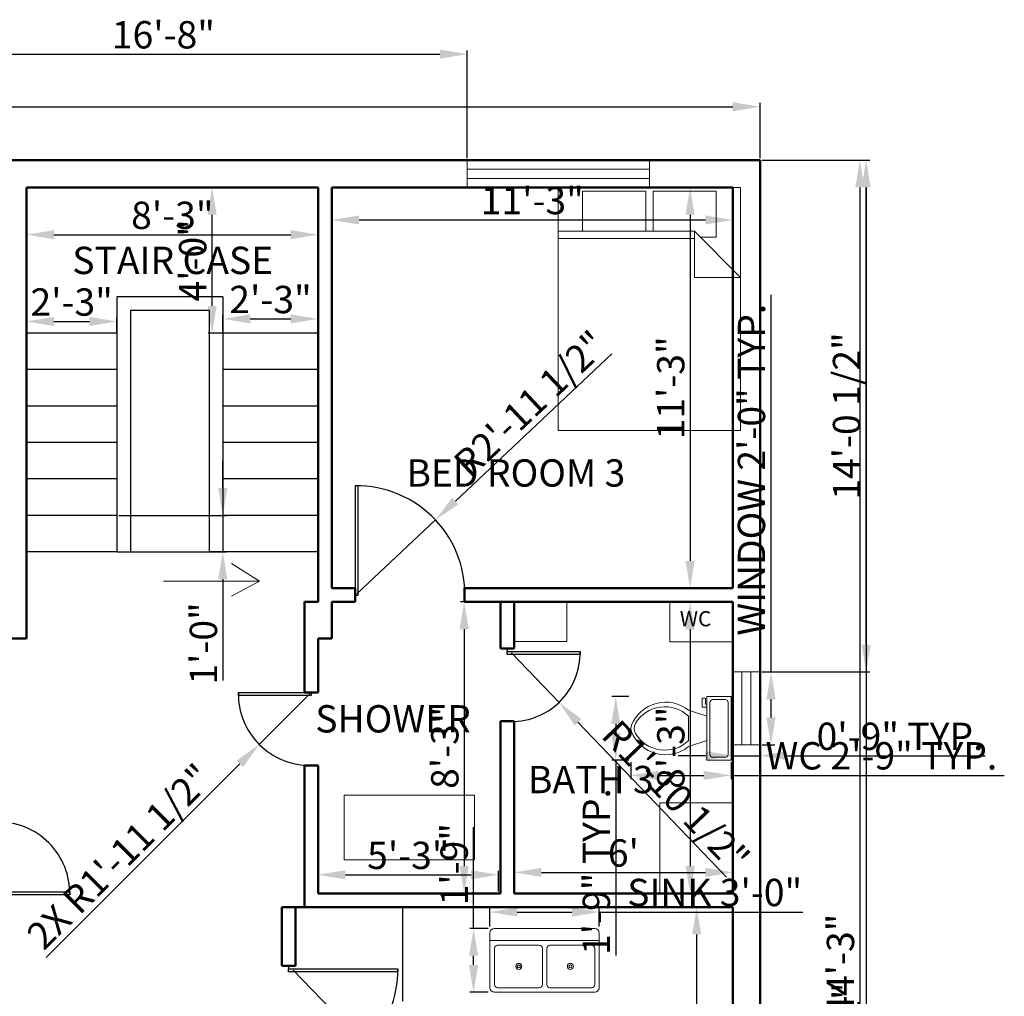
# Model space of a CAD drawing. Units: inches. Extents: x 145135 to 145817, y 90589 to 91373.
# Tile 4 of 4: x 145493 to 145817, y 90973 to 91295. Entities that reach past the tile are written whole.
import ezdxf

# ---------------------------------------------------------------- set-up
doc = ezdxf.new("R2010")
doc.units = ezdxf.units.IN
for name, color, linetype, lineweight in [('A-ANNO-DIMS', 2, 'Continuous', 18), ('A-ANNO-SYMB', 2, 'Continuous', 18), ('A-ANNO-TEXT', 7, 'Continuous', 18), ('A-AREA-IDEN', 7, 'Continuous', 25), ('A-DOOR', 3, 'Continuous', 25), ('A-FLOR-CASE', 8, 'Continuous', 25), ('A-FLOR-FIXT', 9, 'Continuous', 18), ('A-FLOR-STRS', 7, 'Continuous', 25), ('A-FURN', 8, 'Continuous', 18), ('A-GLAZ', 4, 'Continuous', 18), ('A-WALL', 7, 'Continuous', 50)]:
    doc.layers.add(name, color=color, linetype=linetype, lineweight=lineweight)
doc.styles.get("Standard").update_dxf_attribs({"font": 'arial.ttf'})
doc.dimstyles.new('ISO-25', dxfattribs={"dimtxt": 9, "dimasz": 9, "dimexe": 1.25, "dimexo": 0.625, "dimtad": 1, "dimdec": 1, "dimrnd": 9, "dimlunit": 3, "dimtxsty": 'Standard', "dimcen": 2.5, "dimadec": 0, "dimazin": 0, "dimtfac": 1, "dimtdec": 1, "dimtmove": 0, "dimatfit": 3, "dimfxl": 1, "dimarcsym": 0})

# ---------------------------------------------------------------- blocks, each defined once
blk = doc.blocks.new('*D1')
at = {"layer": 'A-ANNO-DIMS', "color": 0, "lineweight": -2, "transparency": 16777216}
for p, q in [((145188.93, 91249.14), (145188.93, 91267.35)), ((145197.93, 91266.1), (145727.43, 91266.1)), ((145736.43, 91249.14), (145736.43, 91267.35))]:
    blk.add_line(p, q, dxfattribs=at)
at = {"layer": 'A-ANNO-DIMS', "color": 0, "transparency": 16777216}
for points in [[(145197.93, 91267.6), (145197.93, 91264.6), (145188.93, 91266.1)], [(145727.43, 91267.6), (145727.43, 91264.6), (145736.43, 91266.1)]]:
    blk.add_solid(points, dxfattribs=at)
at = {"layer": 'Defpoints', "color": 0, "transparency": 16777216}
for p in [(145736.43, 91266.1), (145188.93, 91248.52), (145736.43, 91248.52)]:
    blk.add_point(p, dxfattribs=at)
at = {"layer": 'A-ANNO-DIMS', "color": 0, "transparency": 16777216, "insert": (145462.68, 91271.32), "char_height": 9, "attachment_point": 5}
blk.add_mtext('45\'-9"', dxfattribs=at)
blk = doc.blocks.new('*D7')
at = {"layer": 'A-ANNO-DIMS', "color": 0, "lineweight": -2, "transparency": 16777216}
for p, q in [((145494.93, 91238.89), (145494.93, 91222.72)), ((145590.93, 91238.89), (145590.93, 91222.72)), ((145503.93, 91223.97), (145581.93, 91223.97))]:
    blk.add_line(p, q, dxfattribs=at)
at = {"layer": 'A-ANNO-DIMS', "color": 0, "transparency": 16777216}
for points in [[(145503.93, 91225.47), (145503.93, 91222.47), (145494.93, 91223.97)], [(145581.93, 91225.47), (145581.93, 91222.47), (145590.93, 91223.97)]]:
    blk.add_solid(points, dxfattribs=at)
at = {"layer": 'Defpoints', "color": 0, "transparency": 16777216}
for p in [(145494.93, 91239.52), (145590.93, 91239.52), (145590.93, 91223.97)]:
    blk.add_point(p, dxfattribs=at)
at = {"layer": 'A-ANNO-DIMS', "color": 0, "transparency": 16777216, "insert": (145542.93, 91229.19), "char_height": 9, "attachment_point": 5}
blk.add_mtext('8\'-3"', dxfattribs=at)
blk = doc.blocks.new('*D8')
at = {"layer": 'A-ANNO-DIMS', "color": 0, "lineweight": -2, "transparency": 16777216}
for p, q in [((145494.93, 91192.14), (145494.93, 91196.64)), ((145524.65, 91192.14), (145524.65, 91196.64)), ((145503.93, 91195.39), (145515.65, 91195.39))]:
    blk.add_line(p, q, dxfattribs=at)
at = {"layer": 'A-ANNO-DIMS', "color": 0, "transparency": 16777216}
for points in [[(145503.93, 91196.89), (145503.93, 91193.89), (145494.93, 91195.39)], [(145515.65, 91196.89), (145515.65, 91193.89), (145524.65, 91195.39)]]:
    blk.add_solid(points, dxfattribs=at)
at = {"layer": 'Defpoints', "color": 0, "transparency": 16777216}
for p in [(145524.65, 91195.39), (145494.93, 91191.52), (145524.65, 91191.52)]:
    blk.add_point(p, dxfattribs=at)
at = {"layer": 'A-ANNO-DIMS', "color": 0, "transparency": 16777216, "insert": (145509.79, 91200.62), "char_height": 9, "attachment_point": 5}
blk.add_mtext('2\'-3"', dxfattribs=at)
blk = doc.blocks.new('*D9')
at = {"layer": 'A-ANNO-DIMS', "color": 0, "lineweight": -2, "transparency": 16777216}
for p, q in [((145559.57, 91192.14), (145559.57, 91197.49)), ((145568.57, 91196.24), (145581.93, 91196.24)), ((145590.93, 91192.14), (145590.93, 91197.49))]:
    blk.add_line(p, q, dxfattribs=at)
at = {"layer": 'A-ANNO-DIMS', "color": 0, "transparency": 16777216}
for points in [[(145568.57, 91197.74), (145568.57, 91194.74), (145559.57, 91196.24)], [(145581.93, 91197.74), (145581.93, 91194.74), (145590.93, 91196.24)]]:
    blk.add_solid(points, dxfattribs=at)
at = {"layer": 'Defpoints', "color": 0, "transparency": 16777216}
for p in [(145590.93, 91196.24), (145559.57, 91191.52), (145590.93, 91191.52)]:
    blk.add_point(p, dxfattribs=at)
at = {"layer": 'A-ANNO-DIMS', "color": 0, "transparency": 16777216, "insert": (145575.25, 91201.46), "char_height": 9, "attachment_point": 5}
blk.add_mtext('2\'-3"', dxfattribs=at)
blk = doc.blocks.new('*D10')
at = {"layer": 'A-ANNO-DIMS', "color": 0, "lineweight": -2, "transparency": 16777216}
for p, q in [((145595.43, 91238.89), (145595.43, 91227.56)), ((145727.43, 91238.89), (145727.43, 91227.56)), ((145604.43, 91228.81), (145718.43, 91228.81))]:
    blk.add_line(p, q, dxfattribs=at)
at = {"layer": 'A-ANNO-DIMS', "color": 0, "transparency": 16777216}
for points in [[(145604.43, 91230.31), (145604.43, 91227.31), (145595.43, 91228.81)], [(145718.43, 91230.31), (145718.43, 91227.31), (145727.43, 91228.81)]]:
    blk.add_solid(points, dxfattribs=at)
at = {"layer": 'Defpoints', "color": 0, "transparency": 16777216}
for p in [(145595.43, 91239.52), (145727.43, 91239.52), (145727.43, 91228.81)]:
    blk.add_point(p, dxfattribs=at)
at = {"layer": 'A-ANNO-DIMS', "color": 0, "transparency": 16777216, "insert": (145661.43, 91234.03), "char_height": 9, "attachment_point": 5}
blk.add_mtext('11\'-3"', dxfattribs=at)
blk = doc.blocks.new('*D11')
at = {"layer": 'A-ANNO-DIMS', "color": 0, "lineweight": -2, "transparency": 16777216}
for p, q in [((145726.81, 91239.52), (145712.13, 91239.52)), ((145713.38, 91230.52), (145713.38, 91116.52)), ((145726.81, 91107.52), (145712.13, 91107.52))]:
    blk.add_line(p, q, dxfattribs=at)
at = {"layer": 'A-ANNO-DIMS', "color": 0, "transparency": 16777216}
for points in [[(145711.88, 91230.52), (145714.88, 91230.52), (145713.38, 91239.52)], [(145711.88, 91116.52), (145714.88, 91116.52), (145713.38, 91107.52)]]:
    blk.add_solid(points, dxfattribs=at)
at = {"layer": 'Defpoints', "color": 0, "transparency": 16777216}
for p in [(145727.43, 91239.52), (145713.38, 91107.52), (145727.43, 91107.52)]:
    blk.add_point(p, dxfattribs=at)
at = {"layer": 'A-ANNO-DIMS', "color": 0, "transparency": 16777216, "insert": (145708.16, 91173.52), "char_height": 9, "attachment_point": 5, "rotation": 90}
blk.add_mtext('11\'-3"', dxfattribs=at)
blk = doc.blocks.new('*D12')
at = {"layer": 'A-ANNO-DIMS', "color": 0, "lineweight": -2, "transparency": 16777216}
for p, q in [((145726.81, 91103.02), (145712.16, 91103.02)), ((145713.41, 91094.02), (145713.41, 91016.02)), ((145726.81, 91007.02), (145712.16, 91007.02))]:
    blk.add_line(p, q, dxfattribs=at)
at = {"layer": 'A-ANNO-DIMS', "color": 0, "transparency": 16777216}
for points in [[(145711.91, 91094.02), (145714.91, 91094.02), (145713.41, 91103.02)], [(145711.91, 91016.02), (145714.91, 91016.02), (145713.41, 91007.02)]]:
    blk.add_solid(points, dxfattribs=at)
at = {"layer": 'Defpoints', "color": 0, "transparency": 16777216}
for p in [(145727.43, 91103.02), (145713.41, 91007.02), (145727.43, 91007.02)]:
    blk.add_point(p, dxfattribs=at)
at = {"layer": 'A-ANNO-DIMS', "color": 0, "transparency": 16777216, "insert": (145708.19, 91055.02), "char_height": 9, "attachment_point": 5, "rotation": 90}
blk.add_mtext('8\'-3"', dxfattribs=at)
blk = doc.blocks.new('*D13')
at = {"layer": 'A-ANNO-DIMS', "color": 0, "lineweight": -2, "transparency": 16777216}
for p, q in [((145655.43, 91007.64), (145655.43, 91015.22)), ((145727.43, 91007.64), (145727.43, 91015.22)), ((145664.43, 91013.97), (145718.43, 91013.97))]:
    blk.add_line(p, q, dxfattribs=at)
at = {"layer": 'A-ANNO-DIMS', "color": 0, "transparency": 16777216}
for points in [[(145664.43, 91015.47), (145664.43, 91012.47), (145655.43, 91013.97)], [(145718.43, 91015.47), (145718.43, 91012.47), (145727.43, 91013.97)]]:
    blk.add_solid(points, dxfattribs=at)
at = {"layer": 'Defpoints', "color": 0, "transparency": 16777216}
for p in [(145727.43, 91013.97), (145655.43, 91007.02), (145727.43, 91007.02)]:
    blk.add_point(p, dxfattribs=at)
at = {"layer": 'A-ANNO-DIMS', "color": 0, "transparency": 16777216, "insert": (145691.43, 91019.19), "char_height": 9, "attachment_point": 5}
blk.add_mtext("6'", dxfattribs=at)
blk = doc.blocks.new('*D14')
at = {"layer": 'A-ANNO-DIMS', "color": 0, "lineweight": -2, "transparency": 16777216}
for p, q in [((145650.31, 91103.02), (145637.76, 91103.02)), ((145639.01, 91094.02), (145639.01, 91016.02)), ((145650.31, 91007.02), (145637.76, 91007.02))]:
    blk.add_line(p, q, dxfattribs=at)
at = {"layer": 'A-ANNO-DIMS', "color": 0, "transparency": 16777216}
for points in [[(145637.51, 91094.02), (145640.51, 91094.02), (145639.01, 91103.02)], [(145637.51, 91016.02), (145640.51, 91016.02), (145639.01, 91007.02)]]:
    blk.add_solid(points, dxfattribs=at)
at = {"layer": 'Defpoints', "color": 0, "transparency": 16777216}
for p in [(145650.93, 91103.02), (145639.01, 91007.02), (145650.93, 91007.02)]:
    blk.add_point(p, dxfattribs=at)
at = {"layer": 'A-ANNO-DIMS', "color": 0, "transparency": 16777216, "insert": (145633.79, 91055.02), "char_height": 9, "attachment_point": 5, "rotation": 90}
blk.add_mtext('8\'-3"', dxfattribs=at)
blk = doc.blocks.new('*D15')
at = {"layer": 'A-ANNO-DIMS', "color": 0, "lineweight": -2, "transparency": 16777216}
for p, q in [((145590.93, 91007.64), (145590.93, 91014.43)), ((145599.93, 91013.18), (145641.31, 91013.18)), ((145650.31, 91007.64), (145650.31, 91014.43))]:
    blk.add_line(p, q, dxfattribs=at)
at = {"layer": 'A-ANNO-DIMS', "color": 0, "transparency": 16777216}
for points in [[(145599.93, 91014.68), (145599.93, 91011.68), (145590.93, 91013.18)], [(145641.31, 91014.68), (145641.31, 91011.68), (145650.31, 91013.18)]]:
    blk.add_solid(points, dxfattribs=at)
at = {"layer": 'Defpoints', "color": 0, "transparency": 16777216}
for p in [(145650.31, 91013.18), (145590.93, 91007.02), (145650.31, 91007.02)]:
    blk.add_point(p, dxfattribs=at)
at = {"layer": 'A-ANNO-DIMS', "color": 0, "transparency": 16777216, "insert": (145620.62, 91018.41), "char_height": 9, "attachment_point": 5}
blk.add_mtext('5\'-3"', dxfattribs=at)
blk = doc.blocks.new('*D16')
at = {"layer": 'A-ANNO-DIMS', "color": 0, "lineweight": -2, "transparency": 16777216}
for p, q in [((145726.81, 91002.52), (145714.28, 91002.52)), ((145715.53, 90993.52), (145715.53, 90736.31)), ((145726.81, 90727.31), (145714.28, 90727.31))]:
    blk.add_line(p, q, dxfattribs=at)
at = {"layer": 'A-ANNO-DIMS', "color": 0, "transparency": 16777216}
for points in [[(145714.03, 90993.52), (145717.03, 90993.52), (145715.53, 91002.52)], [(145714.03, 90736.31), (145717.03, 90736.31), (145715.53, 90727.31)]]:
    blk.add_solid(points, dxfattribs=at)
at = {"layer": 'Defpoints', "color": 0, "transparency": 16777216}
for p in [(145727.43, 91002.52), (145715.53, 90727.31), (145727.43, 90727.31)]:
    blk.add_point(p, dxfattribs=at)
at = {"layer": 'A-ANNO-DIMS', "color": 0, "transparency": 16777216, "insert": (145710.31, 90864.92), "char_height": 9, "attachment_point": 5, "rotation": 90}
blk.add_mtext('23\'-3"', dxfattribs=at)
blk = doc.blocks.new('*D27')
at = {"layer": 'A-ANNO-DIMS', "color": 0, "lineweight": -2, "transparency": 16777216}
for p, q in [((145737.06, 91248.52), (145770.52, 91248.52)), ((145769.27, 91239.52), (145769.27, 90727.31)), ((145737.06, 90718.31), (145770.52, 90718.31))]:
    blk.add_line(p, q, dxfattribs=at)
at = {"layer": 'A-ANNO-DIMS', "color": 0, "transparency": 16777216}
for points in [[(145767.77, 91239.52), (145770.77, 91239.52), (145769.27, 91248.52)], [(145767.77, 90727.31), (145770.77, 90727.31), (145769.27, 90718.31)]]:
    blk.add_solid(points, dxfattribs=at)
at = {"layer": 'Defpoints', "color": 0, "transparency": 16777216}
for p in [(145736.43, 91248.52), (145736.43, 90718.31), (145769.27, 90718.31)]:
    blk.add_point(p, dxfattribs=at)
at = {"layer": 'A-ANNO-DIMS', "color": 0, "transparency": 16777216, "insert": (145764.05, 90983.42), "char_height": 9, "attachment_point": 5, "rotation": 90}
blk.add_mtext('44\'-3"', dxfattribs=at)
blk = doc.blocks.new('Toilet - top')
for p, q in [((9.5, -6), (9.5, -2)), ((-10, -8.5), (-8, -8.5)), ((-10, -9.5), (-10, -8.5)), ((-7, -9.5), (-10, -9.5)), ((-8, -8.5), (-8, -8)), ((-7, -8), (-7, -9.5)), ((-4, -8), (-6, -14)), ((4, -8), (6, -14)), ((4, -14), (-4, -14))]:
    blk.add_line(p, q)
blk.add_lwpolyline([(10.5, -8), (10.5, 0), (-10.5, 0), (-10.5, -8)], close=True)
for points in [[(-9.5, -2), (-9.5, -6)], [(8.5, -1), (-8.5, -1)], [(-8.5, -7), (8.5, -7)]]:
    blk.add_lwpolyline(points)
for centre, radius, start, end in [((-8.62, -1.88), 0.884, 81.8699, 188.1301), ((8.62, -1.88), 0.884, 351.8699, 98.1301), ((-8.62, -6.12), 0.884, 171.8699, 278.1301), ((8.62, -6.12), 0.884, 261.8699, 8.1301), ((3.52, -21.58), 12.17, 141.4691, 247.9714), ((4.2, -21.82), 11.33, 136.3677, 238.9468), ((-3.52, -21.58), 12.17, 292.0284, 38.5307), ((-4.2, -21.82), 11.33, 301.053, 43.6321), ((0, -27.88), 4, 245.7318, 294.2682), ((0, -29), 4, 254.8605, 285.1395)]:
    blk.add_arc(centre, radius, start, end)
blk = doc.blocks.new('Sink-double - 36 in top')
for p, q in [((-18, -4), (18, -4)), ((-0.75, -18.5), (-0.75, -6.5)), ((0.75, -6.5), (0.75, -18.5))]:
    blk.add_line(p, q)
for points in [[(-16.5, 0), (16.5, 0)], [(-18, -19.5), (-18, -1.5)], [(18, -1.5), (18, -19.5)], [(-15.5, -5.5), (-1.75, -5.5)], [(1.75, -5.5), (15.5, -5.5)], [(-16.5, -18.5), (-16.5, -6.5)], [(16.5, -6.5), (16.5, -18.5)], [(16.5, -21), (-16.5, -21)], [(-1.75, -19.5), (-15.5, -19.5)], [(15.5, -19.5), (1.75, -19.5)]]:
    blk.add_lwpolyline(points)
for centre, radius in [((-8.5, -12.5), 1), ((-8.5, -12.5), 0.5), ((8.5, -12.5), 1), ((8.5, -12.5), 0.5)]:
    blk.add_circle(centre, radius)
for centre, radius, start, end in [((-16.5, -1.5), 1.5, 90, 180), ((16.5, -1.5), 1.5, 0, 90), ((-15.5, -6.5), 1, 90, 180), ((-1.75, -6.5), 1, 0, 90), ((1.75, -6.5), 1, 90, 180), ((15.5, -6.5), 1, 0, 90), ((-15.5, -18.5), 1, 180, 270), ((-1.75, -18.5), 1, 270, 0), ((1.75, -18.5), 1, 180, 270), ((15.5, -18.5), 1, 270, 0), ((-16.5, -19.5), 1.5, 180, 270), ((16.5, -19.5), 1.5, 270, 0)]:
    blk.add_arc(centre, radius, start, end)
blk = doc.blocks.new('Bed - Queen')
for p, q in [((0, -80.00003), (0, 0)), ((0, 0), (59.99999, 0)), ((59.99999, 0), (59.99999, -80.00003)), ((7.99999, -1.2), (28.79998, -1.2)), ((7.99999, -14.4), (7.99999, -1.2)), ((28.79998, -1.2), (28.79998, -14.4)), ((31.19999, -1.2), (51.99999, -1.2)), ((31.19999, -14.4), (31.19999, -1.2)), ((51.99999, -1.2), (51.99999, -16.4)), ((0, -14.4), (44.8, -14.4)), ((59.99999, -29.6), (44.8, -14.4)), ((44.8, -14.4), (44.8, -29.6)), ((44.8, -16.8), (0, -16.8)), ((51.99999, -16.4), (46.79936, -16.4)), ((44.8, -29.6), (59.99999, -29.6)), ((59.99999, -80.00003), (0, -80.00003))]:
    blk.add_line(p, q)
blk = doc.blocks.new('WIN-60IN')
for p, q in [((0, 9), (0, 0)), ((60, 9), (60, 0)), ((60, 6), (0, 6)), ((60, 3), (0, 3))]:
    blk.add_line(p, q)
blk = doc.blocks.new('WIN-24IN')
for p, q in [((0, 24), (9, 24)), ((3, 0), (3, 24)), ((6, 0), (6, 24)), ((0, 0), (9, 0))]:
    blk.add_line(p, q)
blk = doc.blocks.new('DOOR-SWING-36IN')
for p, q in [((0, 36.03), (0, 35.03)), ((0, 35.03), (36, 35.03)), ((0, 34.03), (0, 35.03)), ((36, 34.03), (0, 34.03)), ((36, 35.03), (36, 34.03))]:
    blk.add_line(p, q)
blk.add_arc((1.47, 34.53), 34.53, 267.5565, 0.8296)
blk = doc.blocks.new('*D42')
at = {"layer": 'A-ANNO-DIMS', "color": 0, "lineweight": -2, "transparency": 16777216}
for p, q in [((145693.86, 91050.24), (145693.86, 91044.66)), ((145726.9, 91050.24), (145726.9, 91044.66)), ((145702.86, 91045.91), (145717.9, 91045.91)), ((145726.9, 91045.91), (145816.82, 91045.91))]:
    blk.add_line(p, q, dxfattribs=at)
at = {"layer": 'A-ANNO-DIMS', "color": 0, "transparency": 16777216}
for points in [[(145702.86, 91047.41), (145702.86, 91044.41), (145693.86, 91045.91)], [(145717.9, 91047.41), (145717.9, 91044.41), (145726.9, 91045.91)]]:
    blk.add_solid(points, dxfattribs=at)
at = {"layer": 'Defpoints', "color": 0, "transparency": 16777216}
for p in [(145693.86, 91050.87), (145726.9, 91050.87), (145726.9, 91045.91)]:
    blk.add_point(p, dxfattribs=at)
at = {"layer": 'A-ANNO-DIMS', "color": 0, "transparency": 16777216, "insert": (145776.36, 91051.19), "char_height": 9, "attachment_point": 5}
blk.add_mtext('WC 2\'-9" TYP.', dxfattribs=at)
blk = doc.blocks.new('*D43')
at = {"layer": 'A-ANNO-DIMS', "color": 0, "lineweight": -2, "transparency": 16777216}
for p, q in [((145693.23, 91071.87), (145687.65, 91071.87)), ((145688.9, 91062.87), (145688.9, 91059.87)), ((145693.23, 91050.87), (145687.65, 91050.87)), ((145688.9, 91050.87), (145688.9, 90986.6))]:
    blk.add_line(p, q, dxfattribs=at)
at = {"layer": 'A-ANNO-DIMS', "color": 0, "transparency": 16777216}
for points in [[(145687.4, 91062.87), (145690.4, 91062.87), (145688.9, 91071.87)], [(145687.4, 91059.87), (145690.4, 91059.87), (145688.9, 91050.87)]]:
    blk.add_solid(points, dxfattribs=at)
at = {"layer": 'Defpoints', "color": 0, "transparency": 16777216}
for p in [(145693.86, 91071.87), (145688.9, 91050.87), (145693.86, 91050.87)]:
    blk.add_point(p, dxfattribs=at)
at = {"layer": 'A-ANNO-DIMS', "color": 0, "transparency": 16777216, "insert": (145683.68, 91014.24), "char_height": 9, "attachment_point": 5, "rotation": 90}
blk.add_mtext('1\'-9" TYP.', dxfattribs=at)
blk = doc.blocks.new('*D46')
at = {"layer": 'A-ANNO-DIMS', "color": 0, "lineweight": -2, "transparency": 16777216}
for p, q in [((145740.03, 91080), (145740.03, 91204.14)), ((145737.06, 91080), (145741.28, 91080)), ((145740.03, 91065), (145740.03, 91071)), ((145737.06, 91056), (145741.28, 91056))]:
    blk.add_line(p, q, dxfattribs=at)
at = {"layer": 'A-ANNO-DIMS', "color": 0, "transparency": 16777216}
for points in [[(145738.53, 91071), (145741.53, 91071), (145740.03, 91080)], [(145738.53, 91065), (145741.53, 91065), (145740.03, 91056)]]:
    blk.add_solid(points, dxfattribs=at)
at = {"layer": 'Defpoints', "color": 0, "transparency": 16777216}
for p in [(145736.43, 91080), (145740.03, 91080), (145736.43, 91056)]:
    blk.add_point(p, dxfattribs=at)
at = {"layer": 'A-ANNO-DIMS', "color": 0, "transparency": 16777216, "insert": (145734.75, 91146.57), "char_height": 9, "attachment_point": 5, "rotation": 90}
blk.add_mtext('WINDOW 2\'-0" TYP.', dxfattribs=at)
blk = doc.blocks.new('*D47')
at = {"layer": 'A-ANNO-DIMS', "color": 0, "lineweight": -2, "transparency": 16777216}
for p, q in [((145727.43, 91055.38), (145727.43, 91051.15)), ((145736.43, 91055.38), (145736.43, 91051.15)), ((145718.43, 91052.4), (145709.43, 91052.4)), ((145727.43, 91052.4), (145736.43, 91052.4)), ((145745.43, 91052.4), (145810.54, 91052.4))]:
    blk.add_line(p, q, dxfattribs=at)
at = {"layer": 'A-ANNO-DIMS', "color": 0, "transparency": 16777216}
for points in [[(145718.43, 91053.9), (145718.43, 91050.9), (145727.43, 91052.4)], [(145745.43, 91053.9), (145745.43, 91050.9), (145736.43, 91052.4)]]:
    blk.add_solid(points, dxfattribs=at)
at = {"layer": 'Defpoints', "color": 0, "transparency": 16777216}
for p in [(145727.43, 91056), (145736.43, 91056), (145736.43, 91052.4)]:
    blk.add_point(p, dxfattribs=at)
at = {"layer": 'A-ANNO-DIMS', "color": 0, "transparency": 16777216, "insert": (145782.49, 91057.62), "char_height": 9, "attachment_point": 5}
blk.add_mtext('0\'-9" TYP.', dxfattribs=at)
blk = doc.blocks.new('*D50')
at = {"layer": 'A-ANNO-DIMS', "color": 0, "lineweight": -2, "transparency": 16777216}
for p, q in [((145647.5, 90996.12), (145647.5, 91002.15)), ((145683.5, 90996.12), (145683.5, 91002.15)), ((145656.5, 91000.9), (145674.5, 91000.9)), ((145683.5, 91000.9), (145750.47, 91000.9))]:
    blk.add_line(p, q, dxfattribs=at)
at = {"layer": 'A-ANNO-DIMS', "color": 0, "transparency": 16777216}
for points in [[(145656.5, 91002.4), (145656.5, 90999.4), (145647.5, 91000.9)], [(145674.5, 91002.4), (145674.5, 90999.4), (145683.5, 91000.9)]]:
    blk.add_solid(points, dxfattribs=at)
at = {"layer": 'Defpoints', "color": 0, "transparency": 16777216}
for p in [(145683.5, 91000.9), (145647.5, 90995.5), (145683.5, 90995.5)]:
    blk.add_point(p, dxfattribs=at)
at = {"layer": 'A-ANNO-DIMS', "color": 0, "transparency": 16777216, "insert": (145721.48, 91006.18), "char_height": 9, "attachment_point": 5}
blk.add_mtext('SINK 3\'-0"', dxfattribs=at)
blk = doc.blocks.new('*D51')
at = {"layer": 'A-ANNO-DIMS', "color": 0, "lineweight": -2, "transparency": 16777216}
for p, q in [((145642.1, 90995.5), (145642.1, 91028.83)), ((145646.88, 90995.5), (145640.85, 90995.5)), ((145642.1, 90983.5), (145642.1, 90986.5)), ((145646.88, 90974.5), (145640.85, 90974.5))]:
    blk.add_line(p, q, dxfattribs=at)
at = {"layer": 'A-ANNO-DIMS', "color": 0, "transparency": 16777216}
for points in [[(145640.6, 90986.5), (145643.6, 90986.5), (145642.1, 90995.5)], [(145640.6, 90983.5), (145643.6, 90983.5), (145642.1, 90974.5)]]:
    blk.add_solid(points, dxfattribs=at)
at = {"layer": 'Defpoints', "color": 0, "transparency": 16777216}
for p in [(145642.1, 90995.5), (145647.5, 90995.5), (145647.5, 90974.5)]:
    blk.add_point(p, dxfattribs=at)
at = {"layer": 'A-ANNO-DIMS', "color": 0, "transparency": 16777216, "insert": (145636.88, 91016.66), "char_height": 9, "attachment_point": 5, "rotation": 90}
blk.add_mtext('1\'-9"', dxfattribs=at)
blk = doc.blocks.new('*D59')
at = {"layer": 'A-ANNO-DIMS', "color": 0, "lineweight": -2, "transparency": 16777216}
for p, q in [((145440, 91249.14), (145440, 91284.67)), ((145640, 91249.14), (145640, 91284.67)), ((145449, 91283.42), (145631, 91283.42))]:
    blk.add_line(p, q, dxfattribs=at)
at = {"layer": 'A-ANNO-DIMS', "color": 0, "transparency": 16777216}
for points in [[(145449, 91284.92), (145449, 91281.92), (145440, 91283.42)], [(145631, 91284.92), (145631, 91281.92), (145640, 91283.42)]]:
    blk.add_solid(points, dxfattribs=at)
at = {"layer": 'Defpoints', "color": 0, "transparency": 16777216}
for p in [(145640, 91283.42), (145440, 91248.52), (145640, 91248.52)]:
    blk.add_point(p, dxfattribs=at)
at = {"layer": 'A-ANNO-DIMS', "color": 0, "transparency": 16777216, "insert": (145540, 91288.64), "char_height": 9, "attachment_point": 5}
blk.add_mtext('16\'-8"', dxfattribs=at)
blk = doc.blocks.new('*D62')
at = {"layer": 'A-ANNO-DIMS', "color": 0, "lineweight": -2, "transparency": 16777216}
for p, q in [((145737.06, 91248.52), (145772.58, 91248.52)), ((145771.33, 91089), (145771.33, 91239.52)), ((145737.06, 91080), (145772.58, 91080))]:
    blk.add_line(p, q, dxfattribs=at)
at = {"layer": 'A-ANNO-DIMS', "color": 0, "transparency": 16777216}
for points in [[(145769.83, 91239.52), (145772.83, 91239.52), (145771.33, 91248.52)], [(145769.83, 91089), (145772.83, 91089), (145771.33, 91080)]]:
    blk.add_solid(points, dxfattribs=at)
at = {"layer": 'Defpoints', "color": 0, "transparency": 16777216}
for p in [(145736.43, 91248.52), (145771.33, 91248.52), (145736.43, 91080)]:
    blk.add_point(p, dxfattribs=at)
at = {"layer": 'A-ANNO-DIMS', "color": 0, "transparency": 16777216, "insert": (145766.06, 91164.26), "char_height": 9, "attachment_point": 5, "rotation": 90}
blk.add_mtext('14\'-0 1/2"', dxfattribs=at)
blk = doc.blocks.new('*D65')
at = {"layer": 'A-ANNO-DIMS', "color": 0, "lineweight": -2, "transparency": 16777216}
for p, q in [((145559.55, 91140.52), (145559.55, 91149.52)), ((145525.28, 91131.52), (145560.8, 91131.52)), ((145559.55, 91131.52), (145559.55, 91119.52)), ((145525.28, 91119.52), (145560.8, 91119.52)), ((145559.55, 91110.52), (145559.55, 91077.19))]:
    blk.add_line(p, q, dxfattribs=at)
at = {"layer": 'A-ANNO-DIMS', "color": 0, "transparency": 16777216}
for points in [[(145558.05, 91140.52), (145561.05, 91140.52), (145559.55, 91131.52)], [(145558.05, 91110.52), (145561.05, 91110.52), (145559.55, 91119.52)]]:
    blk.add_solid(points, dxfattribs=at)
at = {"layer": 'Defpoints', "color": 0, "transparency": 16777216}
for p in [(145524.65, 91131.52), (145524.65, 91119.52), (145559.55, 91119.52)]:
    blk.add_point(p, dxfattribs=at)
at = {"layer": 'A-ANNO-DIMS', "color": 0, "transparency": 16777216, "insert": (145554.33, 91089.35), "char_height": 9, "attachment_point": 5, "rotation": 90}
blk.add_mtext('1\'-0"', dxfattribs=at)
blk = doc.blocks.new('*D66')
at = {"layer": 'A-ANNO-DIMS', "color": 0, "lineweight": -2, "transparency": 16777216}
for p, q in [((145590.31, 91239.52), (145554.78, 91239.52)), ((145556.03, 91200.52), (145556.03, 91230.52)), ((145590.31, 91191.52), (145554.78, 91191.52))]:
    blk.add_line(p, q, dxfattribs=at)
at = {"layer": 'A-ANNO-DIMS', "color": 0, "transparency": 16777216}
for points in [[(145554.53, 91230.52), (145557.53, 91230.52), (145556.03, 91239.52)], [(145554.53, 91200.52), (145557.53, 91200.52), (145556.03, 91191.52)]]:
    blk.add_solid(points, dxfattribs=at)
at = {"layer": 'Defpoints', "color": 0, "transparency": 16777216}
for p in [(145556.03, 91239.52), (145590.93, 91239.52), (145590.93, 91191.52)]:
    blk.add_point(p, dxfattribs=at)
at = {"layer": 'A-ANNO-DIMS', "color": 0, "transparency": 16777216, "insert": (145550.81, 91215.52), "char_height": 9, "attachment_point": 5, "rotation": 90}
blk.add_mtext('4\'-0"', dxfattribs=at)
blk = doc.blocks.new('*D74')
at = {"layer": 'A-ANNO-DIMS', "color": 0, "lineweight": -2, "transparency": 16777216}
for p, q in [((145737.06, 91248.52), (145772.58, 91248.52)), ((145771.33, 91239.52), (145771.33, 90660.88)), ((145551.73, 90651.88), (145772.58, 90651.88))]:
    blk.add_line(p, q, dxfattribs=at)
at = {"layer": 'A-ANNO-DIMS', "color": 0, "transparency": 16777216}
for points in [[(145769.83, 91239.52), (145772.83, 91239.52), (145771.33, 91248.52)], [(145769.83, 90660.88), (145772.83, 90660.88), (145771.33, 90651.88)]]:
    blk.add_solid(points, dxfattribs=at)
at = {"layer": 'Defpoints', "color": 0, "transparency": 16777216}
for p in [(145736.43, 91248.52), (145551.11, 90651.88), (145771.33, 90651.88)]:
    blk.add_point(p, dxfattribs=at)
at = {"layer": 'A-ANNO-DIMS', "color": 0, "transparency": 16777216, "insert": (145766.06, 90950.2), "char_height": 9, "attachment_point": 5, "rotation": 90}
blk.add_mtext('49\'-8 1/2"', dxfattribs=at)
blk = doc.blocks.new('*D75')
at = {"layer": 'A-ANNO-DIMS', "color": 0, "lineweight": -2, "transparency": 16777216}
for p, q in [((145687.62, 91184.73), (145636.1, 91136.24)), ((145603.62, 91105.67), (145629.55, 91130.07))]:
    blk.add_line(p, q, dxfattribs=at)
at = {"layer": 'A-ANNO-DIMS', "color": 0, "transparency": 16777216}
blk.add_solid([(145635.07, 91137.33), (145637.13, 91135.15), (145629.55, 91130.07)], dxfattribs=at)
at = {"layer": 'Defpoints', "color": 0, "transparency": 16777216}
for p in [(145629.55, 91130.07), (145603.62, 91105.67)]:
    blk.add_point(p, dxfattribs=at)
at = {"layer": 'A-ANNO-DIMS', "color": 0, "transparency": 16777216, "insert": (145661.52, 91167.41), "char_height": 9, "attachment_point": 5, "rotation": 43.2644}
blk.add_mtext('R2\'-11 1/2"', dxfattribs=at)
blk = doc.blocks.new('*D78')
at = {"layer": 'A-ANNO-DIMS', "color": 0, "lineweight": -2, "transparency": 16777216}
for p, q in [((145582.66, 90981.74), (145606.73, 90956.98)), ((145675.91, 90885.83), (145613, 90950.53))]:
    blk.add_line(p, q, dxfattribs=at)
at = {"layer": 'A-ANNO-DIMS', "color": 0, "transparency": 16777216}
blk.add_solid([(145614.08, 90951.57), (145611.93, 90949.48), (145606.73, 90956.98)], dxfattribs=at)
at = {"layer": 'Defpoints', "color": 0, "transparency": 16777216}
for p in [(145582.66, 90981.74), (145606.73, 90956.98)]:
    blk.add_point(p, dxfattribs=at)
at = {"layer": 'A-ANNO-DIMS', "color": 0, "transparency": 16777216, "insert": (145651.38, 90918.63), "char_height": 9, "attachment_point": 5, "rotation": 314.1935}
blk.add_mtext('2X R2\'-10 1/2"', dxfattribs=at)
blk = doc.blocks.new('*D79')
at = {"layer": 'A-ANNO-DIMS', "color": 0, "lineweight": -2, "transparency": 16777216}
for p, q in [((145588.18, 91072.72), (145571.56, 91056.1)), ((145501.39, 90985.92), (145565.2, 91049.73))]:
    blk.add_line(p, q, dxfattribs=at)
at = {"layer": 'A-ANNO-DIMS', "color": 0, "transparency": 16777216}
blk.add_solid([(145564.14, 91050.8), (145566.26, 91048.67), (145571.56, 91056.1)], dxfattribs=at)
at = {"layer": 'Defpoints', "color": 0, "transparency": 16777216}
for p in [(145588.18, 91072.72), (145571.56, 91056.1)]:
    blk.add_point(p, dxfattribs=at)
at = {"layer": 'A-ANNO-DIMS', "color": 0, "transparency": 16777216, "insert": (145526.38, 91018.38), "char_height": 9, "attachment_point": 5, "rotation": 45.0008}
blk.add_mtext('2X R1\'-11 1/2"', dxfattribs=at)
blk = doc.blocks.new('*D80')
at = {"layer": 'A-ANNO-DIMS', "color": 0, "lineweight": -2, "transparency": 16777216}
for p, q in [((145654.64, 91086.23), (145670.24, 91069.95)), ((145725.42, 91012.37), (145676.47, 91063.45))]:
    blk.add_line(p, q, dxfattribs=at)
at = {"layer": 'A-ANNO-DIMS', "color": 0, "transparency": 16777216}
blk.add_solid([(145677.55, 91064.49), (145675.39, 91062.41), (145670.24, 91069.95)], dxfattribs=at)
at = {"layer": 'Defpoints', "color": 0, "transparency": 16777216}
for p in [(145654.64, 91086.23), (145670.24, 91069.95)]:
    blk.add_point(p, dxfattribs=at)
at = {"layer": 'A-ANNO-DIMS', "color": 0, "transparency": 16777216, "insert": (145707.87, 91038.31), "char_height": 9, "attachment_point": 5, "rotation": 313.78}
blk.add_mtext('R1\'-10 1/2"', dxfattribs=at)

msp = doc.modelspace()

# ---------------------------------------------------------------- linework, layer by layer
at = {"layer": 'A-ANNO-SYMB'}
for p, q in [((145571.62, 91109.91), (145562.4, 91115.69)), ((145540.03, 91109.91), (145571.62, 91109.91)), ((145571.62, 91109.91), (145562.4, 91104.91))]:
    msp.add_line(p, q, dxfattribs=at)
at = {"layer": 'A-DOOR'}
for p, q in [((145604.12, 91141.27), (145603.12, 91141.27)), ((145603.12, 91141.27), (145603.12, 91107.52)), ((145604.12, 91105.27), (145604.12, 91141.27)), ((145603.12, 91105.27), (145604.12, 91105.27)), ((145653.18, 91087.73), (145653.18, 91086.73)), ((145653.18, 91086.73), (145677.18, 91086.73)), ((145653.18, 91085.73), (145653.18, 91086.73)), ((145677.18, 91086.73), (145677.18, 91085.73)), ((145677.18, 91085.73), (145653.18, 91085.73)), ((145564.68, 91072.22), (145564.68, 91073.22)), ((145564.68, 91073.22), (145588.68, 91073.22)), ((145588.68, 91073.22), (145588.68, 91072.22)), ((145588.68, 91072.22), (145564.68, 91072.22)), ((145485.18, 91007.53), (145509.18, 91007.53)), ((145509.18, 91006.53), (145487.43, 91006.53)), ((145509.18, 91007.53), (145509.18, 91006.53))]:
    msp.add_line(p, q, dxfattribs=at)
for centre, radius, start, end in [((145603.62, 91105.67), 35.6, 355.7238, 90.8048), ((145654.64, 91086.23), 22.55, 266.2916, 1.2707), ((145588.18, 91072.72), 23.51, 178.7811, 271.2189), ((145485.68, 91007.03), 23.51, 358.7811, 91.2189)]:
    msp.add_arc(centre, radius, start, end, dxfattribs=at)
at = {"layer": 'A-FLOR-CASE'}
msp.add_line((145618.84, 90971.55), (145618.84, 91002.52), dxfattribs=at)
at = {"layer": 'A-FLOR-FIXT'}
for p, q in [((145672.75, 91089.96), (145672.75, 91103.02)), ((145706.7, 91089.86), (145706.7, 91103.02)), ((145655.43, 91089.96), (145655.43, 91089.96)), ((145655.43, 91089.96), (145672.75, 91089.96)), ((145727.43, 91089.86), (145706.7, 91089.86)), ((145727.43, 91089.86), (145727.43, 91089.86)), ((145727.43, 91036.84), (145703.44, 91036.84)), ((145703.44, 91036.84), (145703.44, 91007.02))]:
    msp.add_line(p, q, dxfattribs=at)
msp.add_lwpolyline([(145599.45, 91039.36), (145642.36, 91039.36), (145642.36, 91018.12), (145599.45, 91018.12)], close=True, dxfattribs=at)
at = {"layer": 'A-FLOR-STRS'}
for p, q in [((145559.57, 91203.52), (145524.65, 91203.52)), ((145524.65, 91203.52), (145524.65, 91119.52)), ((145559.57, 91203.52), (145559.57, 91119.52)), ((145529.15, 91199.02), (145529.15, 91119.52)), ((145555.07, 91199.02), (145529.15, 91199.02)), ((145555.07, 91199.02), (145555.07, 91119.52)), ((145524.65, 91191.52), (145494.93, 91191.52)), ((145590.93, 91191.52), (145559.57, 91191.52)), ((145524.65, 91179.52), (145494.93, 91179.52)), ((145590.93, 91179.52), (145559.57, 91179.52)), ((145524.65, 91167.52), (145494.93, 91167.52)), ((145590.93, 91167.52), (145559.57, 91167.52)), ((145524.65, 91155.52), (145494.93, 91155.52)), ((145590.93, 91155.52), (145559.57, 91155.52)), ((145524.65, 91143.52), (145494.93, 91143.52)), ((145590.93, 91143.52), (145559.57, 91143.52)), ((145524.65, 91131.52), (145494.93, 91131.52)), ((145590.93, 91131.52), (145559.57, 91131.52)), ((145524.65, 91119.52), (145494.93, 91119.52)), ((145524.65, 91119.52), (145529.15, 91119.52)), ((145559.57, 91119.52), (145555.07, 91119.52)), ((145590.93, 91119.52), (145559.57, 91119.52))]:
    msp.add_line(p, q, dxfattribs=at)
at = {"layer": 'A-WALL'}
for p, q in [((145736.43, 91248.52), (145188.93, 91248.52)), ((145736.43, 90718.31), (145736.43, 91248.52)), ((145494.93, 91091.02), (145494.93, 91239.52)), ((145590.93, 91239.52), (145494.93, 91239.52)), ((145590.93, 91103.02), (145590.93, 91239.52)), ((145727.43, 91239.52), (145595.43, 91239.52)), ((145595.43, 91107.52), (145595.43, 91239.52)), ((145727.43, 91107.52), (145727.43, 91239.52)), ((145603.12, 91107.52), (145595.43, 91107.52)), ((145603.12, 91107.52), (145603.12, 91103.02)), ((145727.43, 91107.52), (145639.12, 91107.52)), ((145639.12, 91107.52), (145639.12, 91103.02)), ((145586.43, 91103.02), (145590.93, 91103.02)), ((145586.43, 91073.22), (145586.43, 91103.02)), ((145595.43, 91091.02), (145595.43, 91103.02)), ((145603.12, 91103.02), (145595.43, 91103.02)), ((145727.43, 91103.02), (145639.12, 91103.02)), ((145650.93, 91087.73), (145650.93, 91103.02)), ((145655.43, 91087.73), (145655.43, 91103.02)), ((145727.43, 91007.02), (145727.43, 91103.02)), ((145494.93, 91091.02), (145487.43, 91091.02)), ((145494.93, 91091.02), (145490.43, 91091.02)), ((145595.43, 91091.02), (145590.93, 91091.02)), ((145595.43, 91091.02), (145590.93, 91091.02)), ((145590.93, 91073.22), (145590.93, 91091.02)), ((145650.93, 91087.73), (145655.43, 91087.73)), ((145586.43, 91073.22), (145590.93, 91073.22)), ((145650.93, 91007.02), (145650.93, 91063.73)), ((145650.93, 91063.73), (145655.43, 91063.73)), ((145655.43, 91007.02), (145655.43, 91063.73)), ((145586.43, 91002.52), (145586.43, 91049.22)), ((145586.43, 91049.22), (145590.93, 91049.22)), ((145590.93, 91007.02), (145590.93, 91049.22)), ((145727.43, 91007.02), (145727.43, 91010.02)), ((145595.43, 91007.02), (145590.93, 91007.02)), ((145650.93, 91007.02), (145595.43, 91007.02)), ((145727.43, 91007.02), (145655.43, 91007.02)), ((145586.43, 91002.52), (145578.93, 91002.52)), ((145578.93, 90983.24), (145578.93, 91002.52)), ((145583.43, 90983.24), (145583.43, 91002.52)), ((145727.43, 91002.52), (145586.43, 91002.52)), ((145727.43, 90727.31), (145727.43, 91002.52)), ((145727.43, 90999.52), (145727.43, 91002.52)), ((145578.93, 90983.24), (145583.43, 90983.24))]:
    msp.add_line(p, q, dxfattribs=at)

# ---------------------------------------------------------------- block references
at = {"layer": 'A-DOOR'}
msp.add_blockref('DOOR-SWING-36IN', (145581.18, 90947.21), dxfattribs=at)
at = {"layer": 'A-FLOR-FIXT', "rotation": 270}
msp.add_blockref('Toilet - top', (145726.9, 91061.37), dxfattribs=at)
at = {"layer": 'A-FLOR-FIXT'}
msp.add_blockref('Sink-double - 36 in top', (145665.5, 90995.5), dxfattribs=at)
at = {"layer": 'A-FURN'}
msp.add_blockref('Bed - Queen', (145670, 91239.52), dxfattribs=at)
at = {"layer": 'A-GLAZ'}
for name, p in [('WIN-60IN', (145640, 91239.52)), ('WIN-24IN', (145727.43, 91056))]:
    msp.add_blockref(name, p, dxfattribs=at)

# ---------------------------------------------------------------- texts
at = {"layer": 'A-ANNO-TEXT', "insert": (145710, 91100), "char_height": 5, "attachment_point": 1}
msp.add_mtext_dynamic_manual_height_columns('WC ', width=20.1144, gutter_width=12.5, heights=[0], dxfattribs=at)
at = {"layer": 'A-AREA-IDEN', "char_height": 9, "attachment_point": 1}
for s, insert in [('STAIR CASE', (145510, 91220)), ('BED ROOM 3', (145620, 91150)), ('SHOWER', (145590, 91069.04)), ('BATH 3', (145660, 91049.04))]:
    msp.add_mtext_dynamic_manual_height_columns(s, width=90, gutter_width=12.5, heights=[0], dxfattribs=dict(at, insert=insert))

# ---------------------------------------------------------------- dimensions: what is measured, and where the dimension line sits
at = {"layer": 'A-ANNO-DIMS'}
for base, p1, p2, override, picture, middle in [((145640, 91283.42), (145440, 91248.52), (145640, 91248.52), {"dimdec": 1, "dimlfac": 1, "dimrnd": 0, "dimzin": 1, "dimdsep": 46, "dimlunit": 4, "dimfrac": 2}, '*D59', (145540, 91288.64)), ((145736.43, 91266.1), (145188.93, 91248.52), (145736.43, 91248.52), {"dimclrd": 0, "dimclre": 0, "dimclrt": 0}, '*D1', (145462.68, 91271.32)), ((145590.93, 91223.97), (145494.93, 91239.52), (145590.93, 91239.52), {"dimclrd": 0, "dimclre": 0, "dimclrt": 0}, '*D7', (145542.93, 91229.19)), ((145727.43, 91228.81), (145595.43, 91239.52), (145727.43, 91239.52), {"dimclrd": 0, "dimclre": 0, "dimclrt": 0}, '*D10', (145661.43, 91234.03)), ((145524.65, 91195.39), (145494.93, 91191.52), (145524.65, 91191.52), {"dimclrd": 0, "dimclre": 0, "dimclrt": 0}, '*D8', (145509.79, 91200.62)), ((145590.93, 91196.24), (145559.57, 91191.52), (145590.93, 91191.52), {"dimclrd": 0, "dimclre": 0, "dimclrt": 0}, '*D9', (145575.25, 91201.46)), ((145650.31, 91013.18), (145590.93, 91007.02), (145650.31, 91007.02), {"dimclrd": 0, "dimclre": 0, "dimclrt": 0}, '*D15', (145620.62, 91018.41)), ((145727.43, 91013.97), (145655.43, 91007.02), (145727.43, 91007.02), {"dimclrd": 0, "dimclre": 0, "dimclrt": 0}, '*D13', (145691.43, 91019.19))]:
    dim = msp.add_linear_dim(base=base, p1=p1, p2=p2, dimstyle='ISO-25', override=override, dxfattribs=at)
    dim.commit()
    dim.dimension.update_dxf_attribs({"geometry": picture, "text_midpoint": middle})
for base, p1, p2, angle, override, picture, middle in [((145771.33, 90651.88), (145736.43, 91248.52), (145551.11, 90651.88), 90, {"dimdec": 1, "dimlfac": 1, "dimrnd": 0, "dimzin": 1, "dimdsep": 46, "dimlunit": 4, "dimfrac": 2}, '*D74', (145766.06, 90950.2)), ((145769.27, 90718.31), (145736.43, 91248.52), (145736.43, 90718.31), 90, {"dimclrd": 0, "dimclre": 0, "dimclrt": 0}, '*D27', (145764.05, 90983.42)), ((145771.33, 91248.52), (145736.43, 91080), (145736.43, 91248.52), 90, {"dimdec": 1, "dimlfac": 1, "dimrnd": 0, "dimzin": 1, "dimdsep": 46, "dimlunit": 4, "dimfrac": 2}, '*D62', (145766.06, 91164.26)), ((145556.03, 91239.52), (145590.93, 91191.52), (145590.93, 91239.52), 90, {"dimdec": 1, "dimlfac": 1, "dimrnd": 0, "dimzin": 1, "dimdsep": 46, "dimlunit": 4, "dimfrac": 2}, '*D66', (145550.81, 91215.52)), ((145713.38, 91107.52), (145727.43, 91239.52), (145727.43, 91107.52), 90, {"dimclrd": 0, "dimclre": 0, "dimclrt": 0}, '*D11', (145708.16, 91173.52)), ((145559.55, 91119.52), (145524.65, 91131.52), (145524.65, 91119.52), 270, {"dimdec": 1, "dimlfac": 1, "dimrnd": 0, "dimzin": 1, "dimdsep": 46, "dimlunit": 4, "dimfrac": 2}, '*D65', (145554.33, 91089.35)), ((145639.01, 91007.02), (145650.93, 91103.02), (145650.93, 91007.02), 90, {"dimclrd": 0, "dimclre": 0, "dimclrt": 0}, '*D14', (145633.79, 91055.02)), ((145713.41, 91007.02), (145727.43, 91103.02), (145727.43, 91007.02), 90, {"dimclrd": 0, "dimclre": 0, "dimclrt": 0}, '*D12', (145708.19, 91055.02)), ((145642.1, 90995.5), (145647.5, 90974.5), (145647.5, 90995.5), 90, {"dimdec": 1, "dimlfac": 1, "dimrnd": 0, "dimzin": 1, "dimdsep": 46, "dimlunit": 4, "dimfrac": 2}, '*D51', (145636.88, 91016.66)), ((145715.53, 90727.31), (145727.43, 91002.52), (145727.43, 90727.31), 90, {"dimclrd": 0, "dimclre": 0, "dimclrt": 0}, '*D16', (145710.31, 90864.92))]:
    dim = msp.add_linear_dim(base=base, p1=p1, p2=p2, angle=angle, dimstyle='ISO-25', override=override, dxfattribs=at)
    dim.commit()
    dim.dimension.update_dxf_attribs({"geometry": picture, "text_midpoint": middle})
for base, p1, p2, angle, text, picture, middle in [((145740.03, 91080), (145736.43, 91056), (145736.43, 91080), 90, 'WINDOW <> TYP.', '*D46', (145734.75, 91146.57)), ((145688.9, 91050.87), (145693.86, 91071.87), (145693.86, 91050.87), 270, '<> TYP.', '*D43', (145683.68, 91014.24))]:
    dim = msp.add_linear_dim(base=base, p1=p1, p2=p2, angle=angle, text=text, dimstyle='ISO-25', override={"dimdec": 1, "dimlfac": 1, "dimrnd": 0, "dimzin": 1, "dimdsep": 46, "dimlunit": 4, "dimfrac": 2}, dxfattribs=at)
    dim.commit()
    dim.dimension.update_dxf_attribs({"geometry": picture, "text_midpoint": middle})
for center, mpoint, picture, middle in [((145603.62, 91105.67), (145629.55, 91130.07), '*D75', (145661.52, 91167.41)), ((145654.64, 91086.23), (145670.24, 91069.95), '*D80', (145707.87, 91038.31))]:
    dim = msp.add_radius_dim(center=center, mpoint=mpoint, dimstyle='ISO-25', override={"dimdec": 1, "dimlfac": 1, "dimrnd": 0, "dimzin": 1, "dimdsep": 46, "dimlunit": 4, "dimfrac": 2}, dxfattribs=at)
    dim.commit()
    dim.dimension.update_dxf_attribs({"geometry": picture, "text_midpoint": middle})
for center, mpoint, picture, middle in [((145588.18, 91072.72), (145571.56, 91056.1), '*D79', (145526.38, 91018.38)), ((145582.66, 90981.74), (145606.73, 90956.98), '*D78', (145651.38, 90918.63))]:
    dim = msp.add_radius_dim(center=center, mpoint=mpoint, text='2X <>', dimstyle='ISO-25', override={"dimdec": 1, "dimlfac": 1, "dimrnd": 0, "dimzin": 1, "dimdsep": 46, "dimlunit": 4, "dimfrac": 2}, dxfattribs=at)
    dim.commit()
    dim.dimension.update_dxf_attribs({"geometry": picture, "text_midpoint": middle})
for base, p1, p2, text, picture, middle in [((145726.9, 91045.91), (145693.86, 91050.87), (145726.9, 91050.87), 'WC <> TYP.', '*D42', (145776.36, 91051.19)), ((145736.43, 91052.4), (145727.43, 91056), (145736.43, 91056), '<> TYP.', '*D47', (145782.49, 91057.62)), ((145683.5, 91000.9), (145647.5, 90995.5), (145683.5, 90995.5), 'SINK <>', '*D50', (145721.48, 91006.18))]:
    dim = msp.add_linear_dim(base=base, p1=p1, p2=p2, text=text, dimstyle='ISO-25', override={"dimdec": 1, "dimlfac": 1, "dimrnd": 0, "dimzin": 1, "dimdsep": 46, "dimlunit": 4, "dimfrac": 2}, dxfattribs=at)
    dim.commit()
    dim.dimension.update_dxf_attribs({"geometry": picture, "text_midpoint": middle})

doc.saveas('drawing.dxf')
